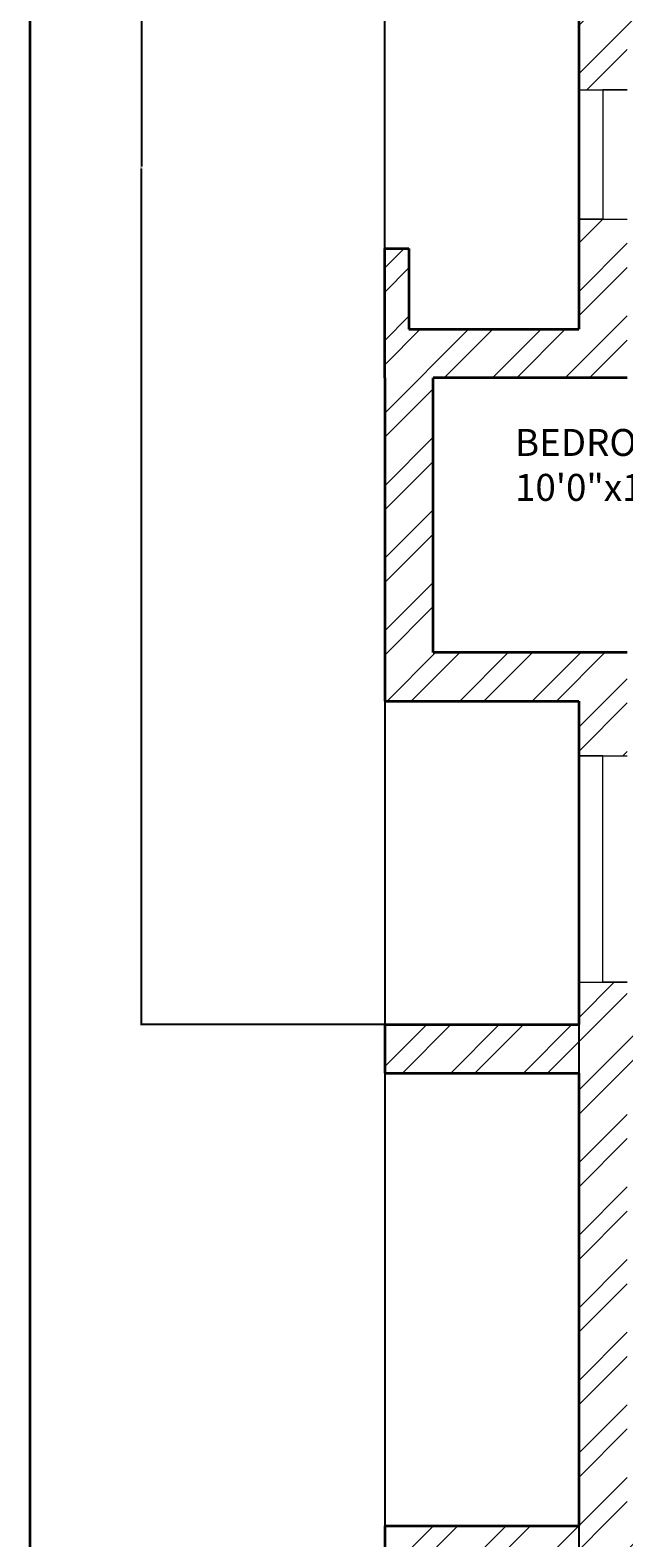
# Model space of a CAD drawing. Units: inches. Extents: x 1513 to 2170, y 1240 to 2288.
# Tile 7 of 10: x 1513 to 1623, y 1801 to 2081. Entities that reach past the tile are written whole.
import ezdxf

# ---------------------------------------------------------------- set-up
doc = ezdxf.new("R2010")
doc.units = ezdxf.units.IN
for name, color, linetype, lineweight in [('A-ANNO-DIMS', 2, 'Continuous', 18), ('A-ANNO-TTLB', 7, 'Continuous', 35), ('A-AREA-IDEN', 7, 'Continuous', 18), ('A-GLAZ', 4, 'Continuous', 18), ('A-WALL', 7, 'Continuous', 35), ('A-WALL-PATT', 252, 'Continuous', 13)]:
    doc.layers.add(name, color=color, linetype=linetype, lineweight=lineweight)
doc.styles.get("Standard").update_dxf_attribs({"font": 'arial.ttf'})
doc.dimstyles.get("Standard").update_dxf_attribs({"dimtxt": 0.18, "dimasz": 0.18, "dimexe": 0.18, "dimexo": 0.0625, "dimgap": 0.09, "dimtad": 0, "dimtih": 1, "dimtoh": 1, "dimdec": 4, "dimzin": 0, "dimdsep": 46, "dimtxsty": 'Standard', "dimcen": 0.09, "dimadec": 0, "dimazin": 0, "dimtfac": 1, "dimtdec": 4, "dimtofl": 0, "dimtmove": 0, "dimatfit": 3, "dimfxl": 1, "dimtolj": 1, "dimtzin": 0, "dimarcsym": 0})

# ---------------------------------------------------------------- blocks, each defined once
blk = doc.blocks.new('WIN-24')
for p, q in [((0, 24), (9, 24)), ((9, 24), (4.5, 24)), ((4.5, 24), (4.5, 0)), ((4.5, 0), (0, 0)), ((0, 0), (9, 0))]:
    blk.add_line(p, q)
blk = doc.blocks.new('*D25')
at = {"layer": 'A-ANNO-DIMS', "color": 0, "lineweight": -2, "transparency": 16777216}
for p, q in [((1578.87, 2040.54), (1578.87, 2259.81)), ((1579.05, 2259.63), (1810.07, 2259.63)), ((2041.67, 2259.63), (1810.65, 2259.63)), ((2041.85, 2040.54), (2041.85, 2259.81))]:
    blk.add_line(p, q, dxfattribs=at)
at = {"layer": 'A-ANNO-DIMS', "color": 0, "transparency": 16777216}
for points in [[(1579.05, 2259.66), (1579.05, 2259.6), (1578.87, 2259.63)], [(2041.67, 2259.66), (2041.67, 2259.6), (2041.85, 2259.63)]]:
    blk.add_solid(points, dxfattribs=at)
at = {"layer": 'Defpoints', "color": 0, "transparency": 16777216}
for p in [(2041.85, 2259.63), (1578.87, 2040.48), (2041.85, 2040.48)]:
    blk.add_point(p, dxfattribs=at)
at = {"layer": 'A-ANNO-DIMS', "color": 0, "transparency": 16777216, "insert": (1810.36, 2259.63), "char_height": 0.18, "attachment_point": 5}
blk.add_mtext('\\A1;463', dxfattribs=at)
blk = doc.blocks.new('*D27')
at = {"layer": 'A-ANNO-DIMS', "color": 0, "lineweight": -2, "transparency": 16777216}
for p, q in [((1578.87, 1956.42), (1578.87, 1344.15)), ((1614.87, 1956.42), (1614.87, 1344.15)), ((1579.05, 1344.33), (1596.65, 1344.33)), ((1614.69, 1344.33), (1597.08, 1344.33))]:
    blk.add_line(p, q, dxfattribs=at)
at = {"layer": 'A-ANNO-DIMS', "color": 0, "transparency": 16777216}
for points in [[(1579.05, 1344.36), (1579.05, 1344.3), (1578.87, 1344.33)], [(1614.69, 1344.36), (1614.69, 1344.3), (1614.87, 1344.33)]]:
    blk.add_solid(points, dxfattribs=at)
at = {"layer": 'Defpoints', "color": 0, "transparency": 16777216}
for p in [(1578.87, 1956.48), (1614.87, 1956.48), (1614.87, 1344.33)]:
    blk.add_point(p, dxfattribs=at)
at = {"layer": 'A-ANNO-DIMS', "color": 0, "transparency": 16777216, "insert": (1596.87, 1344.33), "char_height": 0.18, "attachment_point": 5}
blk.add_mtext('\\A1;36', dxfattribs=at)
blk = doc.blocks.new('*D30')
at = {"layer": 'A-ANNO-DIMS', "color": 0, "lineweight": -2, "transparency": 16777216}
for p, q in [((1614.8, 2214.48), (1533.54, 2214.48)), ((1533.72, 2214.3), (1533.72, 2055.66)), ((1533.72, 1896.66), (1533.72, 2055.3)), ((1578.8, 1896.48), (1533.54, 1896.48))]:
    blk.add_line(p, q, dxfattribs=at)
at = {"layer": 'A-ANNO-DIMS', "color": 0, "transparency": 16777216}
for points in [[(1533.69, 2214.3), (1533.75, 2214.3), (1533.72, 2214.48)], [(1533.69, 1896.66), (1533.75, 1896.66), (1533.72, 1896.48)]]:
    blk.add_solid(points, dxfattribs=at)
at = {"layer": 'Defpoints', "color": 0, "transparency": 16777216}
for p in [(1533.72, 2214.48), (1614.87, 2214.48), (1578.87, 1896.48)]:
    blk.add_point(p, dxfattribs=at)
at = {"layer": 'A-ANNO-DIMS', "color": 0, "transparency": 16777216, "insert": (1533.72, 2055.48), "char_height": 0.18, "attachment_point": 5}
blk.add_mtext('\\A1;318', dxfattribs=at)

msp = doc.modelspace()

# ---------------------------------------------------------------- hatches: boundary and pattern name
at = {"layer": 'A-WALL-PATT'}
h = msp.add_hatch(dxfattribs=at)
h.set_pattern_fill('ANSI32', color=256)
h.paths.add_polyline_path([(2041.852, 1719.48), (2014.852, 1719.48), (2014.852, 1734.444), (2005.852, 1734.444), (2005.852, 1710.48), (2032.852, 1710.48), (2032.852, 1663.98), (1976.619, 1663.98), (1976.619, 1659.48), (2005.852, 1659.48), (2005.852, 1626.27), (2014.852, 1626.27), (2014.852, 1659.48), (2041.852, 1659.48)])
h.paths.add_polyline_path([(1954.521, 1663.98), (1875.357, 1663.98), (1875.357, 1659.48), (1945.852, 1659.48), (1945.852, 1546.98), (1950.352, 1546.98), (2005.852, 1546.98), (2005.852, 1422.48), (1985.47, 1422.48), (1985.47, 1413.48), (2014.852, 1413.48), (2014.852, 1602.27), (2005.852, 1602.27), (2005.852, 1551.48), (1950.352, 1551.48), (1950.352, 1659.48), (1954.521, 1659.48)])
h.paths.add_polyline_path([(1949.47, 1422.48), (1937.366, 1422.48), (1937.366, 1413.48), (1949.47, 1413.48)], flags=0)
h.paths.add_polyline_path([(1937.366, 1422.48), (1908.866, 1422.48), (1908.866, 1546.98), (1805.486, 1546.98), (1805.486, 1542.48), (1904.366, 1542.48), (1904.366, 1451.2), (1897.222, 1451.2), (1897.222, 1442.2), (1904.366, 1442.2), (1904.366, 1422.48), (1904.366, 1413.48), (1904.366, 1389.48), (1908.866, 1389.48), (1908.866, 1413.48), (1932.866, 1413.48), (1932.866, 1389.48), (1937.366, 1389.48)])
h.paths.add_polyline_path([(1830.254, 1442.2), (1844.144, 1442.2), (1844.144, 1451.2), (1830.254, 1451.2), (1821.254, 1451.2), (1821.254, 1422.48), (1766.366, 1422.48), (1766.366, 1542.48), (1770.265, 1542.48), (1770.265, 1546.98), (1758.774, 1546.98), (1758.774, 1544.73), (1758.774, 1542.48), (1761.866, 1542.48), (1761.866, 1389.48), (1779.454, 1389.48), (1779.454, 1398.48), (1770.866, 1398.48), (1770.866, 1413.48), (1830.254, 1413.48)])
h.paths.add_polyline_path([(1686.156, 1451.2), (1677.156, 1451.2), (1677.156, 1422.48), (1623.866, 1422.48), (1623.866, 1460.073), (1614.866, 1460.073), (1614.866, 1413.48), (1686.156, 1413.48)])
h.paths.add_polyline_path([(1761.866, 1422.48), (1686.156, 1422.48), (1686.156, 1413.48), (1761.866, 1413.48)])
h.paths.add_polyline_path([(1623.866, 1542.48), (1688.266, 1542.48), (1688.266, 1544.73), (1688.266, 1546.98), (1623.866, 1546.98), (1623.866, 1560.442), (1614.866, 1560.442), (1614.866, 1520.073), (1619.366, 1520.073), (1623.866, 1520.073)])
h.paths.add_polyline_path([(1623.866, 1600.98), (1715.366, 1600.98), (1715.366, 1546.98), (1711.055, 1546.98), (1711.055, 1542.48), (1719.866, 1542.48), (1726.867, 1542.48), (1726.867, 1544.73), (1726.867, 1546.98), (1719.866, 1546.98), (1719.866, 1600.98), (1719.866, 1608.301), (1717.616, 1608.301), (1715.366, 1608.301), (1715.366, 1605.48), (1623.866, 1605.48), (1623.866, 1620.254), (1614.866, 1620.254), (1614.866, 1584.442), (1623.866, 1584.442)])
h.paths.add_polyline_path([(1623.866, 1659.48), (1715.366, 1659.48), (1715.366, 1629.2), (1719.866, 1629.2), (1719.866, 1659.48), (1767.866, 1659.48), (1767.866, 1629.2), (1772.366, 1629.2), (1772.366, 1663.98), (1578.866, 1663.98), (1578.866, 1661.73), (1578.866, 1659.48), (1578.866, 1635.48), (1583.366, 1635.48), (1583.366, 1654.98), (1614.866, 1654.98), (1614.866, 1644.254), (1619.366, 1644.254), (1623.866, 1644.254)])
h.paths.add_polyline_path([(1788.587, 1798.98), (1788.587, 1803.48), (1623.866, 1803.48), (1623.866, 1887.48), (1829.49, 1887.48), (1829.49, 1891.98), (1829.49, 1896.48), (1748.366, 1896.48), (1743.866, 1896.48), (1623.866, 1896.48), (1623.866, 1904.333), (1619.366, 1904.333), (1614.866, 1904.333), (1614.866, 1896.48), (1578.866, 1896.48), (1578.866, 1887.48), (1614.866, 1887.48), (1614.866, 1803.48), (1578.866, 1803.48), (1578.866, 1794.48), (1626.866, 1794.48), (1788.587, 1794.48)])
h.paths.add_polyline_path([(1635.866, 1794.48), (1626.866, 1794.48), (1626.866, 1763.627), (1631.366, 1763.627), (1635.866, 1763.627)])
h.paths.add_polyline_path([(1635.866, 1703.627), (1626.866, 1703.627), (1626.866, 1663.98), (1635.866, 1663.98)])
h.paths.add_polyline_path([(1587.866, 2016.48), (1614.866, 2016.48), (1623.866, 2016.48), (1707.767, 2016.48), (1707.767, 2018.73), (1707.767, 2020.98), (1706.366, 2020.98), (1706.366, 2025.944), (1701.866, 2025.944), (1701.866, 2020.98), (1623.866, 2020.98), (1623.866, 2045.903), (1614.866, 2045.903), (1614.866, 2025.48), (1583.366, 2025.48), (1583.366, 2040.48), (1578.866, 2040.48), (1578.866, 2016.48), (1578.866, 1956.48), (1614.866, 1956.48), (1614.866, 1946.333), (1623.866, 1946.333), (1623.866, 1965.48), (1587.866, 1965.48)])
h.paths.add_polyline_path([(1748.366, 2016.48), (1748.366, 2025.48), (1743.866, 2025.48), (1739.366, 2025.48), (1739.366, 2020.98), (1738.09, 2020.98), (1738.09, 2016.48), (1743.866, 2016.48), (1743.866, 1896.48), (1748.366, 1896.48)])
h.paths.add_polyline_path([(1746.736, 2085.48), (1623.866, 2085.48), (1623.866, 2205.48), (1657.136, 2205.48), (1657.136, 2214.48), (1614.866, 2214.48), (1614.866, 2069.903), (1623.866, 2069.903), (1623.866, 2080.98), (1683.866, 2080.98), (1701.866, 2080.98), (1701.866, 2046.743), (1706.366, 2046.743), (1706.366, 2080.98), (1746.736, 2080.98)])

# ---------------------------------------------------------------- linework, layer by layer
at = {"layer": 'A-ANNO-TTLB'}
msp.add_lwpolyline([(1513.071, 2287.731), (2170.435, 2287.731), (2170.435, 1239.669), (1513.071, 1239.669)], close=True, dxfattribs=at)
at = {"layer": 'A-GLAZ'}
for p, q in [((1619.366, 1946.333), (1614.866, 1946.333)), ((1614.866, 1946.333), (1623.866, 1946.333)), ((1619.366, 1904.333), (1619.366, 1946.333)), ((1614.866, 1904.333), (1623.866, 1904.333)), ((1623.866, 1904.333), (1619.366, 1904.333))]:
    msp.add_line(p, q, dxfattribs=at)
at = {"layer": 'A-WALL'}
for p, q in [((1614.866, 2214.48), (1614.866, 2025.48)), ((1578.866, 2016.48), (1578.866, 2040.48)), ((1578.866, 2040.48), (1583.366, 2040.48)), ((1583.366, 2040.48), (1583.366, 2025.48)), ((1583.366, 2025.48), (1614.866, 2025.48)), ((1578.866, 2016.48), (1578.866, 1956.48)), ((1614.866, 2016.48), (1587.866, 2016.48)), ((1587.866, 1965.48), (1587.866, 2016.48)), ((1623.866, 2016.48), (1614.866, 2016.48)), ((1623.866, 1965.48), (1587.866, 1965.48)), ((1578.866, 1956.48), (1614.866, 1956.48)), ((1614.866, 1956.48), (1614.866, 1896.48)), ((1578.866, 1896.48), (1614.866, 1896.48)), ((1578.866, 1896.48), (1578.866, 1887.48)), ((1578.866, 1887.48), (1614.866, 1887.48)), ((1614.866, 1887.48), (1614.866, 1803.48)), ((1578.866, 1803.48), (1614.866, 1803.48)), ((1578.866, 1803.48), (1578.866, 1794.48))]:
    msp.add_line(p, q, dxfattribs=at)

# ---------------------------------------------------------------- block references
at = {"layer": 'A-GLAZ'}
msp.add_blockref('WIN-24', (1614.863, 2045.903), dxfattribs=at)

# ---------------------------------------------------------------- texts
at = {"layer": 'A-AREA-IDEN', "insert": (1603.048, 2006.976), "char_height": 5, "attachment_point": 1}
msp.add_mtext_dynamic_manual_height_columns('BEDROOM\\P10\'0"x10\'0"', width=185.75698, gutter_width=12.5, heights=[0], dxfattribs=at)

# ---------------------------------------------------------------- dimensions: what is measured, and where the dimension line sits
at = {"layer": 'A-ANNO-DIMS'}
for base, p1, p2, picture, middle in [((2041.852, 2259.63), (1578.866, 2040.48), (2041.852, 2040.48), '*D25', (1810.359, 2259.63)), ((1614.866, 1344.33), (1578.866, 1956.48), (1614.866, 1956.48), '*D27', (1596.866, 1344.33))]:
    dim = msp.add_linear_dim(base=base, p1=p1, p2=p2, dimstyle='Standard', override={"dimdec": 0, "dimlfac": 1, "dimrnd": 0, "dimzin": 0, "dimdsep": 46, "dimlunit": 2}, dxfattribs=at)
    dim.commit()
    dim.dimension.update_dxf_attribs({"geometry": picture, "text_midpoint": middle})
dim = msp.add_linear_dim(base=(1533.716, 2214.48), p1=(1578.866, 1896.48), p2=(1614.866, 2214.48), angle=90, dimstyle='Standard', override={"dimdec": 0, "dimlfac": 1, "dimrnd": 0, "dimzin": 0, "dimdsep": 46, "dimlunit": 2}, dxfattribs=at)
dim.commit()
dim.dimension.update_dxf_attribs({"geometry": '*D30', "text_midpoint": (1533.716, 2055.48)})

doc.saveas('drawing.dxf')
